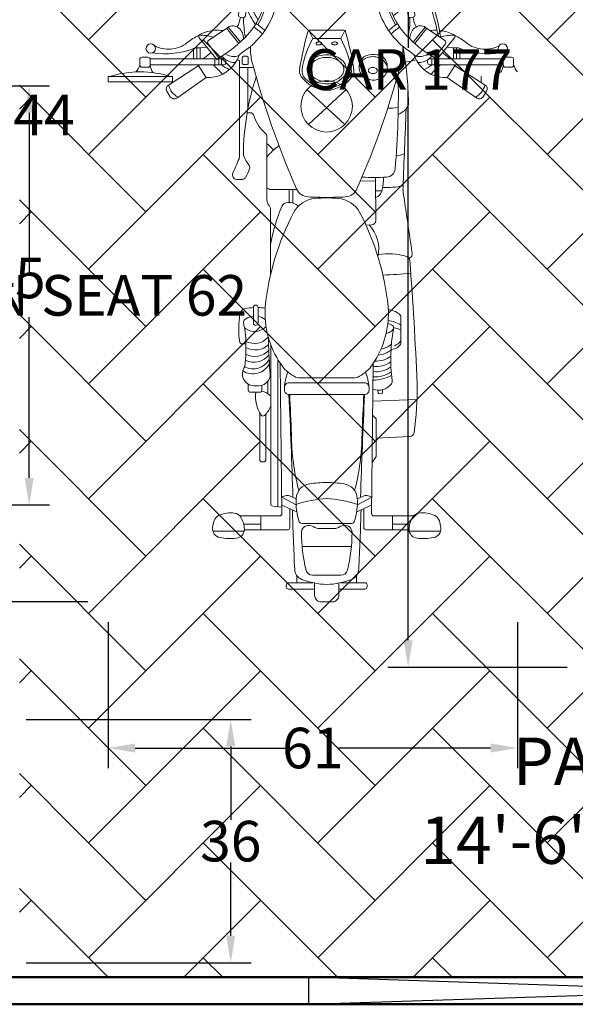
# Model space of a CAD drawing. Units: inches. Extents: x -466983 to 1020, y 324 to 318697.
# Tile 23 of 97: x 814 to 896, y 365 to 511. Entities that reach past the tile are written whole.
import ezdxf

# ---------------------------------------------------------------- set-up
doc = ezdxf.new("R2010")
doc.units = ezdxf.units.IN
doc.header["$MEASUREMENT"] = 0
for name, color, linetype, lineweight in [('A-ANNO-DIMS', 2, 'Continuous', 18), ('A-AREA-IDEN', 7, 'Continuous', 25), ('A-DOOR', 3, 'Continuous', 25), ('A-EQPM-VEHC', 8, 'Continuous', 18), ('A-FLOR-PATT', 252, 'Continuous', 13), ('A-WALL', 7, 'Continuous', 50)]:
    doc.layers.add(name, color=color, linetype=linetype, lineweight=lineweight)
doc.styles.get("Standard").update_dxf_attribs({"font": 'arial.ttf'})
doc.dimstyles.get("Standard").update_dxf_attribs({"dimtxt": 6, "dimasz": 4, "dimexe": 3, "dimexo": 3, "dimgap": 0.09, "dimtad": 0, "dimtih": 1, "dimtoh": 1, "dimdec": 1, "dimzin": 0, "dimdsep": 46, "dimlunit": 3, "dimtxsty": 'Standard', "dimcen": 0.09, "dimadec": 0, "dimazin": 0, "dimtfac": 1, "dimtdec": 1, "dimtofl": 0, "dimtmove": 0, "dimatfit": 3, "dimfxl": 1, "dimtolj": 1, "dimtzin": 0, "dimarcsym": 0})

# ---------------------------------------------------------------- blocks, each defined once
blk = doc.blocks.new('Bike')
for p, q in [((3716.6, 1477), (3739.4, 1477)), ((3715, 1462.6), (3739.4, 1462.6)), ((3715.3, 1469.7), (3739.4, 1469.7)), ((3725.9, 1437.8), (3739.4, 1455.6)), ((3476.2, 1372.3), (3476.2, 1447.6)), ((3479.4, 1371.4), (3479.4, 1449.1)), ((4796.8, 1363.8), (4796.8, 1434.1)), ((3739.4, 1429.3), (3753.1, 1429.3)), ((3739.4, 1420.3), (3753.1, 1420.3)), ((3739.4, 1414.7), (3753.1, 1414.7)), ((3511.5, 1359.9), (3511.5, 1390.3)), ((3668.6, 1399.5), (3702.1, 1372.5)), ((3671.4, 1403.4), (3705.4, 1376.1)), ((3478.1, 1297.1), (3478.1, 1372)), ((3491.8, 1338.1), (3491.8, 1373.1)), ((4502.2, 1381), (4505.8, 1282.1)), ((3511.5, 1346.8), (3511.5, 1327.3)), ((4781.5, 1364.7), (4781.5, 1326.4)), ((3478.1, 1338.1), (3495.7, 1338.1)), ((3505.6, 1338.1), (3511.5, 1338.1)), ((4762.6, 1326.4), (4793.8, 1326.4)), ((4035.1, 1288.5), (4035.1, 1302.5)), ((3491.8, 1289.6), (3530.3, 1289.6)), ((4012.9, 1254.3), (4013.4, 1288.4)), ((4721.1, 1279.7), (4737.7, 1247.6)), ((4738.5, 1279.5), (4753.4, 1246.1)), ((3106.7, 1249.4), (3106.7, 1240.7)), ((3129.5, 1249.4), (3129.5, 1240.7)), ((3460.4, 1251.7), (3510.3, 1251.7)), ((3517.1, 1251.6), (3529.2, 1251.6)), ((3542.4, 1251.6), (3546.2, 1251.6)), ((4896.6, 1245.7), (4912.2, 1245.7)), ((3808.6, 1222.8), (3886.6, 1138)), ((3808.6, 1134.7), (3886.6, 1219.4)), ((3489.4, 1202.6), (3538.3, 1202.6)), ((3489.4, 1155.3), (3538.3, 1155.3)), ((3676.5, 1138.6), (3694.4, 1147.6)), ((3106.7, 1108.5), (3106.7, 1117.1)), ((3129.5, 1108.5), (3129.5, 1117.1)), ((3460.4, 1106.2), (3510.3, 1106.2)), ((3517.1, 1106.2), (3529.2, 1106.2)), ((3542.4, 1106.2), (3546.2, 1106.2)), ((4032.4, 1103.3), (4062.6, 1103.3)), ((4721.1, 1078.2), (4737.7, 1110.3)), ((4738.5, 1078.4), (4753.4, 1111.8)), ((4896.6, 1112.2), (4912.2, 1112.2)), ((4032.4, 1094.9), (4061.1, 1094.9)), ((3478.1, 1060.8), (3478.1, 985.9)), ((3491.8, 1068.2), (3530.3, 1068.2)), ((4412.5, 1069.2), (4742.2, 1069.2)), ((4461.5, 1046.8), (4489.1, 1046.8)), ((3478.1, 1019.8), (3500.2, 1019.8)), ((3491.8, 1019.8), (3491.8, 984.8)), ((3500.1, 1019.8), (3511.5, 1019.8)), ((3511.5, 996.5), (3511.5, 1030.6)), ((3758.9, 1015.1), (3758.9, 983.2)), ((4762.6, 1031.4), (4793.8, 1031.4)), ((4781.5, 993.1), (4781.5, 1031.4)), ((3511.5, 998), (3511.5, 967.6)), ((3758.9, 1002.4), (3851.5, 1002.4)), ((4796.8, 994.1), (4796.8, 923.8)), ((3476.2, 985.5), (3476.2, 910.3)), ((3479.4, 986.4), (3479.4, 908.8)), ((3668.6, 958.4), (3702.1, 985.4)), ((3671.4, 954.4), (3705.4, 981.8)), ((3739.4, 943.1), (3753.1, 943.1)), ((3739.4, 937.5), (3753.1, 937.5)), ((3739.4, 928.6), (3753.1, 928.6)), ((3725.9, 920.1), (3739.4, 902.3)), ((3755, 891.8), (3781.3, 909.1)), ((3715, 895.3), (3739.4, 895.3)), ((3715.3, 888.2), (3739.4, 888.2)), ((3716.6, 880.8), (3739.4, 880.8))]:
    blk.add_line(p, q)
for points in [[(3736.2, 1579.4), (3736.2, 1592.7, -0.414214), (3741.2, 1597.7), (3753.5, 1597.7, -0.414214), (3758.5, 1592.7), (3758.5, 1579.4, -0.414214), (3753.5, 1574.4), (3741.2, 1574.4, -0.414214)], [(3506.4, 1438.1, 0.044309), (3491.8, 1448.2, 0.12965), (3486.9, 1449.5), (3482.3, 1449.5, 0.116215), (3477.8, 1448.5, 0.026021), (3471.7, 1445, 0.256394), (3464.8, 1432.4), (3464.8, 1387.3, 0.252462), (3471.5, 1374.8, 0.012105), (3473, 1373.9, 0.288965), (3494.3, 1374.5, 0.06955), (3510.2, 1388.8, 0.177075), (3517.3, 1408.1), (3517.3, 1415, 0.223082)], [(4811.1, 1418.6, 0.390363), (4789.3, 1434.7, 0.055736), (4773.5, 1431.2, 0.196303), (4762.1, 1421.2, 0.154867), (4756.5, 1385.4, 0.215074), (4765.4, 1371.6, 0.140504), (4792.5, 1363.4, 0.387027), (4812.7, 1381.2, 0.07489)], [(3764.2, 1314.8, 0.116891), (3754.2, 1313.4, 0.104306), (3744.8, 1307.4, 0.090357), (3738.3, 1297.9, 0.08248), (3735, 1285.8, 0.08248), (3735.8, 1273.2, 0.090357), (3740.4, 1262.7, 0.104306), (3748.4, 1254.9, 0.116891), (3757.9, 1251.6, 0.116891), (3767.8, 1252.9, 0.104306), (3777.2, 1259, 0.090357), (3783.8, 1268.4, 0.08248), (3787.1, 1280.6, 0.08248), (3786.2, 1293.1, 0.090357), (3781.7, 1303.7, 0.104306), (3773.6, 1311.5, 0.116891)], [(4294.6, 1316.7, 0.093727), (4084.2, 1253.4, 0.26048), (4052.1, 1204.4, 0.011277), (4050.8, 1178.9, 0.011277), (4052.1, 1153.4, 0.26048), (4084.2, 1104.5, 0.093727), (4294.6, 1041.2, 0.168473), (4422.7, 1075.8, 0.123184), (4450.3, 1105.7, 0.12588), (4454, 1120.1), (4454, 1178.9), (4454, 1237.8, 0.12588), (4450.3, 1252.2, 0.123184), (4422.7, 1282.1, 0.168473)], [(3564.6, 1285.6, 0.137096), (3561.5, 1285.3, 0.107007), (3558.1, 1283.1, 0.081077), (3555.6, 1279.7, 0.06906), (3554.1, 1275, 0.06906), (3553.9, 1270, 0.081077), (3554.9, 1265.9, 0.107007), (3557.3, 1262.7, 0.137096), (3560.1, 1261.3, 0.137096), (3563.3, 1261.6, 0.107007), (3566.7, 1263.8, 0.081077), (3569.1, 1267.2, 0.06906), (3570.7, 1271.9, 0.06906), (3570.9, 1276.8, 0.081077), (3569.8, 1280.9, 0.107007), (3567.5, 1284.2, 0.137096)], [(3766.3, 1292.1, 0.136763), (3763.8, 1291.6, 0.10699), (3761.3, 1289.5, 0.081228), (3759.7, 1286.4, 0.069255), (3758.9, 1282.5, 0.069255), (3759.2, 1278.5, 0.081228), (3760.5, 1275.3, 0.10699), (3762.8, 1272.9, 0.136763), (3765.2, 1272.1, 0.136763), (3767.7, 1272.7, 0.10699), (3770.2, 1274.8, 0.081228), (3771.8, 1277.8, 0.069255), (3772.6, 1281.8, 0.069255), (3772.3, 1285.8, 0.081228), (3771, 1288.9, 0.10699), (3768.7, 1291.3, 0.136763)], [(3409.7, 1259.3, 0.088306), (3400.8, 1259.5, 0.265111), (3393, 1253.4, 0.077673), (3375.4, 1178.9, 0.077673), (3393, 1104.4, 0.265111), (3400.8, 1098.3, 0.088306), (3409.7, 1098.6, 0.355135), (3417.6, 1108.4), (3417.6, 1178.9), (3417.6, 1249.5, 0.355135)], [(3556.1, 1227.7), (3556.1, 1236.5, -0.414214), (3561.1, 1241.5), (3613.3, 1241.5, -0.414214), (3618.3, 1236.5), (3618.3, 1227.7, -0.414214), (3613.3, 1222.7), (3561.1, 1222.7, -0.414214)], [(3779.6, 1236, 0.198787), (3764.7, 1239.7, 0.033352), (3679.3, 1221.3, 0.334742), (3675.6, 1216.5), (3675.6, 1178.9), (3675.6, 1141.3, 0.334742), (3679.3, 1136.5, 0.033352), (3764.7, 1118.1, 0.198787), (3779.6, 1121.9, 0.220896), (3810.5, 1178.9, 0.220896)], [(4687.9, 1178.9, 0.027846), (4690.9, 1140.7, 0.357798), (4723.4, 1110.4, 0.096715), (4776.1, 1117.3, 0.32255), (4779.5, 1122.1), (4779.5, 1178.9), (4779.5, 1235.8, 0.32255), (4776.1, 1240.6, 0.096715), (4723.4, 1247.4, 0.357798), (4690.9, 1217.2, 0.027846)], [(4790.8, 1178.9), (4790.8, 1160.8, -0.145244), (4788.4, 1152.6, 0.168226), (4784.2, 1135.8, 0.389485), (4799.2, 1122.2, 0.058321), (4883.9, 1132.5, 0.346221), (4895.4, 1147.1), (4895.4, 1178.9), (4895.4, 1210.8, 0.346221), (4883.9, 1225.4, 0.058321), (4799.2, 1235.7, 0.389485), (4784.2, 1222, 0.168226), (4788.4, 1205.3, -0.145244), (4790.8, 1197.1)], [(3730.6, 1178.9, 0.074545), (3733.2, 1161.5, 0.085152), (3740.2, 1147.8, 0.106245), (3751.3, 1138, 0.128192), (3763.2, 1134.9, 0.128192), (3775.2, 1138, 0.106245), (3786.3, 1147.8, 0.085152), (3793.3, 1161.5, 0.074545), (3795.9, 1178.9, 0.074545), (3793.3, 1196.3, 0.085152), (3786.3, 1210.1, 0.106245), (3775.2, 1219.9, 0.128192), (3763.2, 1223, 0.128192), (3751.3, 1219.9, 0.106245), (3740.2, 1210.1, 0.085152), (3733.2, 1196.3, 0.074545)], [(3736.5, 1178.9, 0.070978), (3738.7, 1163.7, 0.082547), (3744.4, 1151.7, 0.106804), (3753.7, 1143.1, 0.13387), (3763.6, 1140.5, 0.13387), (3773.4, 1143.1, 0.106804), (3782.7, 1151.7, 0.082547), (3788.4, 1163.7, 0.070978), (3790.6, 1178.9, 0.070978), (3788.4, 1194.2, 0.082547), (3782.7, 1206.1, 0.106804), (3773.4, 1214.7, 0.13387), (3763.6, 1217.4, 0.13387), (3753.7, 1214.7, 0.106804), (3744.4, 1206.1, 0.082547), (3738.7, 1194.2, 0.070978)], [(3705.3, 1202.8, 0.162281), (3704.1, 1202.4, 0.10607), (3702.8, 1200.9, 0.070038), (3702.1, 1199, 0.056281), (3701.8, 1196.5, 0.056281), (3702.1, 1194, 0.070038), (3702.8, 1192.1, 0.10607), (3704.1, 1190.7, 0.162281), (3705.3, 1190.3, 0.162281), (3706.5, 1190.7, 0.10607), (3707.7, 1192.1, 0.070038), (3708.4, 1194, 0.056281), (3708.7, 1196.5, 0.056281), (3708.4, 1199, 0.070038), (3707.7, 1200.9, 0.10607), (3706.5, 1202.4, 0.162281)], [(3705.3, 1155.1, 0.162281), (3706.5, 1155.5, 0.10607), (3707.7, 1156.9, 0.070038), (3708.4, 1158.8, 0.056281), (3708.7, 1161.4, 0.056281), (3708.4, 1163.9, 0.070038), (3707.7, 1165.8, 0.10607), (3706.5, 1167.2, 0.162281), (3705.3, 1167.6, 0.162281), (3704.1, 1167.2, 0.10607), (3702.8, 1165.8, 0.070038), (3702.1, 1163.9, 0.056281), (3701.8, 1161.4, 0.056281), (3702.1, 1158.8, 0.070038), (3702.8, 1156.9, 0.10607), (3704.1, 1155.5, 0.162281)], [(3556.1, 1130.2), (3556.1, 1121.4, 0.414214), (3561.1, 1116.4), (3613.3, 1116.4, 0.414214), (3618.3, 1121.4), (3618.3, 1130.2, 0.414214), (3613.3, 1135.2), (3561.1, 1135.2, 0.414214)], [(3564.6, 1072.3, 0.137096), (3567.5, 1073.7, 0.107007), (3569.8, 1077, 0.081077), (3570.9, 1081, 0.06906), (3570.7, 1086, 0.06906), (3569.1, 1090.7, 0.081077), (3566.7, 1094.1, 0.107007), (3563.3, 1096.3, 0.137096), (3560.1, 1096.6, 0.137096), (3557.3, 1095.2, 0.107007), (3554.9, 1091.9, 0.081077), (3553.9, 1087.9, 0.06906), (3554.1, 1082.9, 0.06906), (3555.6, 1078.2, 0.081077), (3558.1, 1074.8, 0.107007), (3561.5, 1072.6, 0.137096)], [(4291, 1019.6), (4291, 1020, -0.414214), (4296, 1025), (4331.3, 1025, -0.414214), (4336.3, 1020), (4336.3, 1019.6, -0.414214), (4331.3, 1014.6), (4296, 1014.6, -0.414214)], [(3734.1, 992.8), (3734.1, 999.9, -0.414214), (3737.1, 1002.9), (3749.4, 1002.9, -0.414214), (3752.4, 999.9), (3752.4, 992.8, -0.414214), (3749.4, 989.8), (3737.1, 989.8, -0.414214)], [(4812.7, 976.7, 0.387027), (4792.5, 994.5, 0.140504), (4765.4, 986.3, 0.215074), (4756.5, 972.5, 0.154867), (4762.1, 936.7, 0.196303), (4773.5, 926.7, 0.055736), (4789.3, 923.2, 0.390363), (4811.1, 939.2, 0.07489)], [(3517.3, 942.8), (3517.3, 949.8, 0.177075), (3510.2, 969.1, 0.06955), (3494.3, 983.4, 0.288965), (3473, 984, 0.012105), (3471.5, 983.1, 0.252462), (3464.8, 970.6), (3464.8, 925.5, 0.256394), (3471.7, 912.9, 0.026021), (3477.8, 909.4, 0.116215), (3482.3, 908.4), (3486.9, 908.4, 0.12965), (3491.8, 909.7, 0.044309), (3506.4, 919.8, 0.223082)], [(3780.1, 689), (3790, 689, 0.414214), (3791, 690), (3791, 832.2, 0.414214), (3790, 833.2), (3780.1, 833.2, 0.414214), (3779.1, 832.2), (3779.1, 690, 0.414214)], [(3736.2, 778.4), (3736.2, 765.2, 0.414214), (3741.2, 760.2), (3753.5, 760.2, 0.414214), (3758.5, 765.2), (3758.5, 778.4, 0.414214), (3753.5, 783.4), (3741.2, 783.4, 0.414214)]]:
    blk.add_lwpolyline(points, format="xyb", close=True)
for points in [[(3713.9, 1447.6, 0.022793), (3715.3, 1473.8, 0.136), (3726.4, 1569.3)], [(3739.4, 1574.8), (3739.4, 1409.9, 0.414214), (3744.4, 1404.9), (3748.1, 1404.9, 0.414214), (3753.1, 1409.9), (3753.1, 1574.4)], [(3691, 1434, -0.079005), (3686.9, 1465, -0.05973), (3703.5, 1491.3, 0.159047), (3718.1, 1528.9, 0.126021), (3710.9, 1564.4)], [(3753.1, 1463), (3798.3, 1533.8, -0.40834), (3811.9, 1536.9), (3824.4, 1529.3, -0.431541), (3827.4, 1515.1), (3781.3, 1448.7), (3755, 1466.1)], [(3779.1, 1525.7, 0.414214), (3780.1, 1524.7), (3790, 1524.7, 0.414214), (3791, 1525.7)], [(3742, 1424.6), (3692.9, 1464.8, 0.483058), (3685.2, 1463.1, 0.088789), (3676.2, 1431.5)], [(3692.5, 1434.2, 0.096183), (3535.6, 1379.4, 0.22037), (3483.3, 1302.5)], [(3579.8, 1394.4), (3579.8, 1391.2, 0.349421), (3583.7, 1386.3, 0.057073), (3613.1, 1383, 0.413662), (3618.1, 1388), (3618.1, 1433.9, 0.414214), (3613.1, 1438.9), (3594.8, 1438.9, 0.414214), (3579.8, 1423.9), (3579.8, 1401.9)], [(3737.5, 1420.6), (3706.2, 1444.8, 0.431039), (3699, 1443.7), (3669.3, 1400.5, 0.337774), (3670.5, 1376.2, 0.230362), (3695.1, 1365.4)], [(3741.3, 1406, -0.159938), (3748.2, 1383.3, 0.280919), (3781.3, 1448.7)], [(3688.4, 1428.2, 0.089404), (3543.1, 1375.3, 0.184983), (3494.2, 1313)], [(3537.7, 1208.8, -0.564837), (3504.3, 1226.3, -0.102735), (3505.1, 1243.5, -0.140154), (3509.2, 1250.6, -0.082892), (3602.5, 1314.4, -0.053437), (3615.6, 1318.8, 0.151196), (3693.3, 1363.4, 0.070423), (3739.4, 1423.8)], [(3603.7, 1241.5), (3603.7, 1249.5, -0.101252), (3612.6, 1280.5, -0.13244), (3623.3, 1292, -0.090169), (3638.2, 1297.9, 0.164837), (3725.3, 1368), (3729.9, 1373.3, 0.174158), (3734.8, 1386, 0.159727), (3728.6, 1406.2)], [(3454.1, 1241.7, -0.235435), (3643.3, 1361.2, 0.410863), (3647.8, 1366.7, 0.044254), (3646.7, 1372.8, 0.360214), (3641.5, 1376.5, 0.253572), (3442.6, 1247.5)], [(3851.8, 1356.9, 0.001252), (4028.5, 1349.8, 0.046276), (4039.5, 1350.4, 0.000101), (4174.5, 1370.4, -0.314799), (4184.8, 1365.3), (4186, 1363.2)], [(4589, 1290), (4585.2, 1365.1, 0.35984), (4576.7, 1374.5, 0.038725), (4466.4, 1381.4, 0.009033), (4191, 1365, 0.303597), (4182.3, 1358.1, 0.12706), (4178.4, 1294.5)], [(4421.3, 1283), (4757.5, 1279.3, 0.417467), (4762.6, 1284.3), (4762.6, 1373.6)], [(3711.6, 1008.5, 0.070303), (3742.4, 1010.7, 0.039628), (4030.9, 1111.4, 0.282444), (4048.7, 1137.2, 0.015247), (4049.8, 1178.9, 0.015247), (4048.7, 1220.7, 0.282444), (4030.9, 1246.5, 0.039628), (3742.4, 1347.2, 0.070303), (3711.6, 1349.4)], [(3864.3, 1338.9, 0.080734), (3852.8, 1356, 0.212509), (3837.8, 1362.2, 0.038096), (3711.9, 1349.7)], [(4301, 1317, -0.138428), (4310.6, 1341, -0.233155), (4318.5, 1344.9), (4374.8, 1344.9, -0.216687), (4382.4, 1341.5, -0.156826), (4390.4, 1322.8)], [(4746.4, 1261.7), (4788.8, 1261.7, 0.414214), (4793.8, 1266.7), (4793.8, 1363.4)], [(4004.7, 1257.8, 0.018709), (4004.5, 1312.9, 0.375923), (3986.3, 1332, 0.029426), (3773.7, 1338.7)], [(4354.1, 1312.1, 0.056144), (4350.9, 1321, 0.085082), (4347.3, 1326.2, 0.153535), (4342.4, 1328.6, 0.197677), (4338.3, 1327.7, 0.1268), (4335.1, 1324, 0.072333), (4332.4, 1315.8, 0.051836)], [(4479.1, 1282.4, 0.326046), (4467.3, 1323.7, 0.2025), (4459.8, 1325.7, -0.079204), (4344.5, 1328.2)], [(3611.5, 1313.2, 0.084453), (3515.3, 1250, 0.185223), (3510.6, 1240.3, 0.080228), (3511.8, 1223.9, 0.449113), (3537, 1214.3)], [(3627.1, 1321.9, 0.043315), (3622.3, 1319.9, 0.279952), (3580.6, 1252.4), (3580.6, 1241.5)], [(3757.9, 1314.5, 0.058653), (3749, 1313.6, 0.314496), (3730.4, 1291.7, 0.11242), (3732.3, 1267.9, 0.161441), (3739.7, 1257.7, 0.088312), (3749.1, 1253.2, 0.094137), (3758.6, 1251.5)], [(4050.2, 1288.6, 0.000873), (4050.2, 1288.7, 0.265813), (4035.8, 1302.3, 0.056152), (4004.7, 1306.3)], [(4481.3, 1293.5), (4486.7, 1293.8, 0.420229), (4488.6, 1296), (4488.1, 1302.3, 0.415516), (4485.9, 1304.1), (4480.3, 1303.7)], [(3284.5, 1297.1), (3100.9, 1297.1, 0.226605), (3093.1, 1293.4, 0.400758), (3096.5, 1251.9, 0.183413), (3103.2, 1249.4), (3281.2, 1249.4)], [(3324.7, 1299.2, 0.006041), (3316.2, 1299.3), (3290.7, 1299.3, 0.172401), (3284.4, 1297, 0.450807), (3282.4, 1248.2, 0.193514), (3289.3, 1245.4), (3311, 1245.4, 0.017498), (3327.2, 1245.7)], [(3334.2, 1289.8, 0.161741), (3331.4, 1296.9, 0.157572), (3325.7, 1299, 0.171418), (3320.4, 1297.4, 0.113331), (3316.3, 1292.6, 0.072079), (3313, 1283.4, 0.055689), (3312.2, 1273.3, 0.053775), (3313.6, 1263, 0.064911), (3317.3, 1253.4, 0.09694), (3321.7, 1248.1, 0.155824), (3327.4, 1245.9, 0.172526), (3332.7, 1247.4, 0.151352), (3336.2, 1251.6)], [(3392.3, 1251.6), (3324.6, 1251.6, -0.26356), (3320.3, 1254, -0.214715), (3316.5, 1286.3, -0.327171), (3321.3, 1289.8), (3471.6, 1289.8)], [(3570.1, 1297.2, 0.144644), (3549.1, 1299.6, 0.369621), (3527.5, 1282.5, 0.036315), (3527.3, 1266.8)], [(3555, 1300.1, 0.253732), (3540.7, 1282.5, 0.012512), (3540.3, 1277.1)], [(3541.9, 1253.9, 0.31484), (3574.9, 1255.4, 0.193965), (3580.6, 1265, 0.061634), (3581.2, 1286.2, 0.219833), (3576.9, 1293.4, 0.014528), (3575.1, 1294.6)], [(4005.1, 1288.4), (4101.4, 1288.7, -0.407202), (4111.4, 1279), (4111.7, 1266.7)], [(4720.8, 1279.7, 0.108929), (4717, 1269, 0.145286), (4718.3, 1260.6), (4724.6, 1247.5)], [(3527.8, 1096.9, -0.055925), (3533.1, 1120.5, 0.050281), (3539.5, 1178.9, 0.050281), (3533.1, 1237.4, -0.055925), (3527.8, 1261)], [(3540.3, 1086.8, -0.079272), (3546.2, 1120.5, 0.050281), (3552.6, 1178.9, 0.050281), (3546.2, 1237.4, -0.079272), (3540.3, 1271.1)], [(4721.2, 1103.2, 0.004418), (4491.2, 1094.2, -0.414214), (4481.2, 1084.2), (4474.7, 1084.2, -0.414214), (4464.7, 1094.2), (4464.7, 1178.9), (4464.7, 1263.7, -0.414214), (4474.7, 1273.7), (4481.2, 1273.7, -0.414214), (4491.2, 1263.7)], [(4491.2, 1094.2), (4491.2, 1178.9), (4491.2, 1263.7, 0.004418), (4721.2, 1254.7)], [(4705.9, 1241.5, 0.063368), (4580, 1258, -0.001705), (4491.2, 1262)], [(4926.4, 1206.2), (4926.4, 1264.5, 0.414214), (4921.4, 1269.5), (4917.2, 1269.5, 0.414214), (4912.2, 1264.5), (4912.2, 1210.4)], [(3388.2, 1117.1), (3071.5, 1117.1, -0.369002), (3046.8, 1138.2, -0.033307), (3043.1, 1178.9, -0.033307), (3046.8, 1219.6, -0.369002), (3071.5, 1240.7), (3388.2, 1240.7)], [(3392.7, 1239.9, 0.062968), (3380.1, 1178.9, 0.062968), (3392.7, 1118)], [(3416.3, 1103.3, 0.231711), (3486.9, 1148.9, 0.086055), (3494.3, 1178.9, 0.086055), (3486.9, 1209, 0.231711), (3416.3, 1254.6)], [(3694.4, 1210.2), (3694.4, 1178.9), (3694.4, 1147.6, 0.084607), (3762, 1124, 0.24184), (3783.8, 1130.9, 0.177565), (3806.3, 1178.9, 0.177565), (3783.8, 1227, 0.24184), (3762, 1233.9, 0.084607), (3694.4, 1210.2), (3676.5, 1219.3)], [(4736.9, 1247.6, 0.067766), (4724, 1178.9, 0.067766), (4736.9, 1110.2)], [(4748.9, 1102, 0.004183), (4881.9, 1107.1, 0.304225), (4904.8, 1123, 0.085326), (4916.2, 1178.9, 0.085326), (4904.8, 1234.8, 0.304225), (4881.9, 1250.8, 0.004183), (4748.9, 1255.9)], [(3551.4, 1136.8, 0.036141), (3554.8, 1178.9, 0.036141), (3551.4, 1221.1)], [(3608.7, 1135.2, -0.133909), (3615.9, 1165.1, 0.12166), (3620.2, 1178.9, 0.12166), (3615.9, 1192.7, -0.133909), (3608.7, 1222.7)], [(4913.1, 1206.2), (4940.3, 1206.2, -0.414214), (4955.3, 1191.2), (4955.3, 1178.9), (4955.3, 1166.7, -0.414214), (4940.3, 1151.7), (4913.1, 1151.7)], [(3537.7, 1149.1, 0.564837), (3504.3, 1131.6, 0.102735), (3505.1, 1114.4, 0.140154), (3509.2, 1107.3, 0.082892), (3602.5, 1043.5, 0.053437), (3615.6, 1039, -0.151196), (3693.3, 994.4, -0.070423), (3739.4, 934)], [(4912.2, 1147.5), (4912.2, 1093.4, 0.414214), (4917.2, 1088.4), (4921.4, 1088.4, 0.414214), (4926.4, 1093.4), (4926.4, 1151.7)], [(3537, 1143.6, 0.449113), (3511.8, 1134, 0.080228), (3510.6, 1117.6, 0.185223), (3515.3, 1107.9, 0.084453), (3611.5, 1044.6)], [(3281.2, 1108.5), (3103.2, 1108.5, 0.183413), (3096.5, 1106, 0.400758), (3093.1, 1064.5, 0.226605), (3100.9, 1060.7), (3284.5, 1060.7)], [(3327.2, 1112.1, 0.017498), (3311, 1112.5), (3289.3, 1112.5, 0.193514), (3282.4, 1109.7, 0.450807), (3284.4, 1060.8, 0.172401), (3290.7, 1058.6), (3316.2, 1058.6, 0.006041), (3324.7, 1058.7)], [(3336.2, 1106.3, 0.151352), (3332.7, 1110.5, 0.172526), (3327.4, 1112, 0.155824), (3321.7, 1109.8, 0.09694), (3317.3, 1104.4, 0.064911), (3313.6, 1094.9, 0.053775), (3312.2, 1084.5, 0.055689), (3313, 1074.5, 0.072079), (3316.3, 1065.2, 0.113331), (3320.4, 1060.5, 0.171418), (3325.7, 1058.8, 0.157572), (3331.4, 1060.9, 0.161741), (3334.2, 1068.1)], [(3392.3, 1106.3), (3324.6, 1106.3, 0.26356), (3320.3, 1103.8, 0.214715), (3316.5, 1071.6, 0.327171), (3321.3, 1068.1), (3471.6, 1068.1)], [(3442.6, 1110.3, 0.253572), (3641.5, 981.4, 0.360214), (3646.7, 985.1, 0.044254), (3647.8, 991.2, 0.410863), (3643.3, 996.6, -0.235435), (3454.1, 1116.2)], [(3575.1, 1063.2, 0.014528), (3576.9, 1064.4, 0.219833), (3581.2, 1071.7, 0.061634), (3580.6, 1092.8, 0.193965), (3574.9, 1102.5, 0.31484), (3541.9, 1104)], [(3580.6, 1116.4), (3580.6, 1105.5, 0.279952), (3622.3, 1037.9, 0.043315), (3627.1, 1036)], [(3728.6, 951.6, 0.159727), (3734.8, 971.9, 0.174158), (3729.9, 984.5), (3725.3, 989.8, 0.164837), (3638.2, 1059.9, -0.090169), (3623.3, 1065.9, -0.13244), (3612.6, 1077.3, -0.101252), (3603.7, 1108.3), (3603.7, 1116.4)], [(4032.4, 1112), (4032.4, 1054.3, -0.140419), (4030.9, 1049), (4028.4, 1045)], [(4069.3, 1115.5, 0.182977), (4061, 1091.7, 0.292151), (4070, 1078.3, 0.060635), (4155.6, 1053.1)], [(4491.2, 1095.9, -0.001705), (4580, 1099.9, 0.063368), (4705.9, 1116.4)], [(4724.6, 1110.4), (4718.3, 1097.3, 0.145286), (4717, 1088.8, 0.108929), (4720.8, 1078.2)], [(3527.3, 1091.1, 0.036315), (3527.5, 1075.3, 0.369621), (3549.1, 1058.3, 0.144644), (3570.1, 1060.7)], [(3540.3, 1080.8, 0.012512), (3540.7, 1075.3, 0.253732), (3555, 1057.8)], [(4793.8, 994.5), (4793.8, 1091.2, 0.414214), (4788.8, 1096.2), (4746.4, 1096.2)], [(4379.8, 1053.5), (4735.9, 1053.5, 0.378085), (4740.8, 1057.9), (4743.4, 1078.4)], [(4762.6, 984.3), (4762.6, 1073.6, 0.417467), (4757.5, 1078.6), (4421.3, 1074.8)], [(3860.2, 1000.8), (3860.2, 1006.9, -0.339938), (3867.7, 1016.5, 0.159134), (3905.8, 1041.3, -0.226589), (3913.5, 1045), (4055.5, 1045, 0.174252), (4068.2, 1049.6), (4069.7, 1050.8, -0.174252), (4076, 1053.1), (4223.9, 1053.1)], [(4316, 1014.6, 0.114491), (4321.5, 997.6, 0.239101), (4329.2, 992.8, 0.103983), (4339, 994, 0.167173), (4344.1, 997.9, 0.363558), (4338.9, 1042.9)], [(4338.2, 993.7, -0.040508), (4365, 997.7, -0.03842), (4428.6, 995.4, 0.607774), (4471.6, 1015.9), (4471.5, 1027, 0.485016), (4437.8, 1051.6, -0.00298), (4362, 1047.8)], [(4485.9, 1020.1, 0.170118), (4536.9, 1031.7, 0.477675), (4537.8, 1039.4, 0.09469), (4517.6, 1053.5)], [(4532, 1028.9), (4637, 1028.9, 0.414214), (4642, 1033.9), (4642, 1037.6, 0.414214), (4637, 1042.6), (4534.5, 1042.6)], [(3741.8, 978.4, 0.005304), (3743.1, 983.2), (3959.4, 983.2, -0.102096), (3963.4, 982.4, 0.00244), (3995.8, 968.6, 0.501027), (4009.6, 976.7, 0.054221), (4009.7, 990, 0.228934), (4005.1, 997.3, 0.079407), (3985, 1006, 0.239312), (3976.1, 1004, -0.075874), (3957.8, 993, -0.0999), (3953.9, 992.2, -0.077513), (3779.8, 1020.9)], [(4296.5, 1014.6, 0.031683), (4298.6, 996.5, 0.319342), (4310.9, 984.3, 0.078645), (4373.6, 984.1, 0.339222), (4377.8, 988.5, 0.096684), (4377, 998)], [(4470.4, 1033.9), (4480.9, 1033.9, -0.414214), (4485.9, 1028.9), (4485.9, 1008.2, -0.414214), (4480.9, 1003.2), (4467.9, 1003.2)], [(3695.1, 992.5, 0.230362), (3670.5, 981.6, 0.337774), (3669.3, 957.4), (3699, 914.2, 0.431039), (3706.2, 913.1), (3737.5, 937.3)], [(3593, 990.1, 0.064082), (3595.5, 956.1, 0.274699), (3598.9, 952.4, 0.213807), (3609.1, 953.6, 0.217468), (3611.4, 957.1, 0.038755), (3614, 985.1)], [(3753.1, 894.9), (3798.3, 824.1, 0.40834), (3811.9, 820.9), (3824.4, 828.5, 0.431541), (3827.4, 842.8), (3781.3, 909.1, 0.280919), (3748.2, 974.6, -0.159938), (3741.3, 951.9)], [(3753.1, 783.4), (3753.1, 948, 0.414214), (3748.1, 953), (3744.4, 953, 0.414214), (3739.4, 948), (3739.4, 783.1)], [(3676.4, 947.1, 0.047742), (3675.9, 929.4), (3675.9, 929.3, 0.096803), (3685.2, 894.8, 0.483058), (3692.9, 893.1), (3742, 933.3)], [(3691.4, 925.3, 0.082553), (3686.9, 892.9, 0.05973), (3703.5, 866.6, -0.159047), (3718.1, 829, -0.126021), (3710.9, 793.5)], [(3726.4, 788.6, 0.136), (3715.3, 884.1, 0.022793), (3713.9, 910.3)]]:
    blk.add_lwpolyline(points, format="xyb")
for points in [[(4537.3, 1281.8), (4545.1, 1290), (4630.1, 1290), (4643.2, 1280.6)], [(3392.7, 1105.3), (3392.7, 1178.9), (3392.7, 1252.6)], [(4831, 1234.2), (4831, 1178.9), (4831, 1123.7)], [(3050.6, 1229.4), (2939.7, 1229.4), (2802.2, 1229.4), (2775.9, 1217), (2775.9, 1164.4)], [(2776, 1217), (2957.8, 1217), (3046.4, 1217)], [(3580.6, 1222.7), (3580.6, 1178.9), (3580.6, 1135.2)], [(3603.7, 1222.7), (3603.7, 1178.9), (3603.7, 1135.2)], [(3050.6, 1128.5), (2939.7, 1128.5), (2802.2, 1128.5), (2775.9, 1140.9), (2775.9, 1193.5)], [(2776, 1140.9), (2957.8, 1140.9), (3046.4, 1140.9)]]:
    blk.add_lwpolyline(points)
for centre, radius in [((3716.6, 1573.3), 10.6), ((3845.9, 1178.7), 57.6), ((3716.6, 784.6), 10.6)]:
    blk.add_circle(centre, radius)
for centre, radius, start, end in [((3741.5, 1637.1), 41.2, 286.9888, 312.0372), ((3749, 1534.6), 40.1, 57.3492, 83.449), ((3788.9, 1493.4), 40.9, 27.2359, 77.1495), ((3908.5, 1569.9), 206.8, 221.2614, 229.5793), ((3769, 1422), 93.3, 177.6075, 186.9102), ((3710.3, 1384.2), 37.9, 39.0272, 51.9723), ((3680.5, 1359.4), 91.4, 24.0671, 37.4396), ((3939.5, 1465.4), 346.6, 193.685, 195.7923), ((3803.7, 1426.1), 199.4, 192.4698, 195.6556), ((3774.2, 1434.7), 169, 197.8118, 201.3124), ((3639.5, 1433), 61.1, 276.8609, 298.2339), ((3711.2, 1436.9), 65.1, 287.813, 304.5915), ((3515.3, 1317.4), 234.8, 9.2486, 15.3175), ((3597.6, 1291.6), 626.2, 1.209, 6.9337), ((3939.5, 1465.4), 346.6, 198.4449, 204.6334), ((3803.7, 1426.1), 199.4, 200.2574, 210.9013), ((3774.2, 1434.7), 169, 206.8349, 219.1999), ((3649, 1152.2), 213.1, 78.6059, 90.3415), ((3923.3, 1335), 33.4, 359.0902, 32.2964), ((3841.7, 1313.3), 185.9, 357.1486, 11.3635), ((4387.6, 1310.4), 62.2, 146.2979, 174.4306), ((4408.7, 1315.7), 68.7, 154.8594, 169.0097), ((4355, 1321.8), 28.2, 18.3548, 54.9232), ((3584.9, 1462.7), 151.5, 283.3715, 301.3249), ((3834.7, 1458.1), 211.7, 214.8443, 221.5826), ((3842.4, 1463.3), 211.7, 214.9067, 221.5218), ((3733.5, 1322.4), 116.7, 356.6367, 8.2567), ((4337, 1290.1), 53.6, 11.0089, 38.6482), ((4349.2, 1289.8), 53.6, 4.6068, 37.9011), ((4362.7, 1290.1), 53.6, 356.0108, 36.9065), ((4374.9, 1290.1), 53.6, 352.3592, 36.9849), ((4386.5, 1290.4), 53.6, 351.8913, 37.1496), ((4388.7, 1287), 62.9, 356.0657, 35.4453), ((4364.1, 1281), 94.8, 0.9619, 27.161), ((3664.1, 1323.1), 52.9, 190.2344, 217.1371), ((3671.6, 1327), 52.9, 189.3206, 216.9338), ((3343.1, 1272.2), 42, 139.9272, 219.6749), ((3435.7, 1263), 41.9, 140.3451, 189.8858), ((3483.9, 1259.5), 69.2, 154.0504, 182.4153), ((3479.7, 1264.6), 43.4, 144.5037, 201.1055), ((3538.9, 1269.4), 45, 153.363, 203.2549), ((3783.3, 1235.1), 174.2, 162.8434, 177.8981), ((4165.8, 1215.8), 79.7, 77.8259, 132.9545), ((4481.9, 1161.8), 112.1, 93.7127, 111.5258), ((3394.4, 1259.4), 95.6, 334.4456, 355.3484), ((3397.9, 1258.1), 95.6, 333.0513, 356.1505), ((3585.6, 1280.9), 68.9, 237.8956, 265.8204), ((3394.4, 1098.5), 95.6, 4.6516, 25.5544), ((3397.9, 1099.8), 95.6, 3.8495, 26.9487), ((3585.6, 1077), 68.9, 94.1796, 122.1044), ((3343.1, 1085.7), 42, 140.3251, 220.0728), ((3435.7, 1094.9), 41.9, 170.1142, 219.6549), ((3479.7, 1093.3), 43.4, 158.8945, 215.4963), ((3538.9, 1088.4), 45, 156.7451, 206.637), ((3783.3, 1122.7), 174.2, 182.1019, 197.1566), ((3483.9, 1098.4), 69.2, 177.5847, 205.9496), ((4481.9, 1196.1), 112.1, 248.4742, 266.2873), ((3664.1, 1034.8), 52.9, 142.8629, 169.7656), ((3671.6, 1030.9), 52.9, 143.0662, 170.6794), ((4082.7, 908.2), 205.4, 132.3055, 138.2462), ((4027.2, 1133.1), 111.1, 213.3859, 232.4739), ((3584.9, 895.2), 151.5, 58.6751, 76.6285), ((3834.7, 899.8), 211.7, 138.4174, 145.1557), ((4440.3, 1021.4), 143.9, 172.1779, 178.584), ((4355.4, 1018.1), 39.6, 144.2076, 169.9356), ((4336.5, 1017), 40.3, 331.7508, 49.9014), ((4349.2, 1019.2), 42.2, 329.8767, 44.2278), ((4363.9, 1017.8), 42.2, 331.3167, 48.0597), ((4376.7, 1015.8), 42.2, 333.1337, 53.4177), ((4391.4, 1013.8), 42.2, 333.4944, 59.7642), ((4402.5, 1013.1), 42.2, 327.9971, 63.0183), ((4528.9, 1021.1), 47.3, 136.8041, 165.0837), ((3586.6, 1121.8), 117.1, 275.9386, 304.5183), ((3566.8, 1150.4), 162.3, 291.2356, 306.3114), ((3842.4, 894.6), 211.7, 138.4782, 145.0933), ((3649, 1205.7), 213.1, 269.6585, 281.3941), ((3639.5, 924.8), 61.1, 61.7661, 83.1391), ((3711.2, 921), 65.1, 55.4085, 72.187), ((3710.3, 973.7), 37.9, 308.0277, 320.9728), ((3680.5, 998.5), 91.4, 322.5604, 335.9329), ((3908.5, 788), 206.8, 130.4207, 138.7386), ((3788.9, 864.5), 40.9, 282.8505, 332.7641), ((4007, 761.1), 238.1, 163.1793, 196.8207), ((3749, 823.3), 40.1, 276.551, 302.6508), ((3741.5, 720.8), 41.2, 47.9628, 73.0112)]:
    blk.add_arc(centre, radius, start, end)
blk = doc.blocks.new('*D93')
at = {"layer": 'A-ANNO-DIMS', "color": 0, "lineweight": -2, "transparency": 16777216}
for p, q in [((808.97, 500.78), (818.27, 500.78)), ((815.27, 496.78), (815.27, 472.97)), ((815.27, 442.78), (815.27, 466.58)), ((808.97, 438.78), (818.27, 438.78))]:
    blk.add_line(p, q, dxfattribs=at)
at = {"layer": 'A-ANNO-DIMS', "color": 0, "transparency": 16777216}
for points in [[(814.6, 496.78), (815.93, 496.78), (815.27, 500.78)], [(814.6, 442.78), (815.93, 442.78), (815.27, 438.78)]]:
    blk.add_solid(points, dxfattribs=at)
at = {"layer": 'Defpoints', "color": 0, "transparency": 16777216}
for p in [(805.97, 500.78), (815.27, 500.78), (805.97, 438.78)]:
    blk.add_point(p, dxfattribs=at)
at = {"layer": 'A-ANNO-DIMS', "color": 0, "transparency": 16777216, "insert": (815.27, 469.78), "char_height": 6, "attachment_point": 5}
blk.add_mtext('\\A1;GARDEN SEAT 62', dxfattribs=at)
blk = doc.blocks.new('*D95')
at = {"layer": 'A-ANNO-DIMS', "color": 0, "lineweight": -2, "transparency": 16777216}
for p, q in [((894.88, 591.6), (868.36, 591.6)), ((871.36, 587.6), (871.36, 506.38)), ((871.36, 418.77), (871.36, 499.99)), ((894.88, 414.77), (868.36, 414.77))]:
    blk.add_line(p, q, dxfattribs=at)
at = {"layer": 'A-ANNO-DIMS', "color": 0, "transparency": 16777216}
for points in [[(870.69, 587.6), (872.03, 587.6), (871.36, 591.6)], [(870.69, 418.77), (872.03, 418.77), (871.36, 414.77)]]:
    blk.add_solid(points, dxfattribs=at)
at = {"layer": 'Defpoints', "color": 0, "transparency": 16777216}
for p in [(897.88, 591.6), (871.36, 414.77), (897.88, 414.77)]:
    blk.add_point(p, dxfattribs=at)
at = {"layer": 'A-ANNO-DIMS', "color": 0, "transparency": 16777216, "insert": (871.36, 503.18), "char_height": 6, "attachment_point": 5}
blk.add_mtext('\\A1;CAR 177', dxfattribs=at)
blk = doc.blocks.new('*D97')
at = {"layer": 'A-ANNO-DIMS', "color": 0, "lineweight": -2, "transparency": 16777216}
for p, q in [((823.93, 568.44), (802.33, 568.44)), ((805.33, 564.44), (805.33, 499.55)), ((805.33, 428.44), (805.33, 493.34)), ((823.93, 424.44), (802.33, 424.44))]:
    blk.add_line(p, q, dxfattribs=at)
at = {"layer": 'A-ANNO-DIMS', "color": 0, "transparency": 16777216}
for points in [[(804.66, 564.44), (806, 564.44), (805.33, 568.44)], [(804.66, 428.44), (806, 428.44), (805.33, 424.44)]]:
    blk.add_solid(points, dxfattribs=at)
at = {"layer": 'Defpoints', "color": 0, "transparency": 16777216}
for p in [(826.93, 568.44), (805.33, 424.44), (826.93, 424.44)]:
    blk.add_point(p, dxfattribs=at)
at = {"layer": 'A-ANNO-DIMS', "color": 0, "transparency": 16777216, "insert": (805.33, 496.44), "char_height": 6, "attachment_point": 5}
blk.add_mtext('\\A1;BIKE 144', dxfattribs=at)
blk = doc.blocks.new('*D98')
at = {"layer": 'A-ANNO-DIMS', "color": 0, "lineweight": -2, "transparency": 16777216}
for p, q in [((826.93, 421.44), (826.93, 399.84)), ((887.55, 421.44), (887.55, 399.84)), ((830.93, 402.84), (853.42, 402.84)), ((883.55, 402.84), (861.07, 402.84))]:
    blk.add_line(p, q, dxfattribs=at)
at = {"layer": 'A-ANNO-DIMS', "color": 0, "transparency": 16777216}
for points in [[(830.93, 403.51), (830.93, 402.17), (826.93, 402.84)], [(883.55, 403.51), (883.55, 402.17), (887.55, 402.84)]]:
    blk.add_solid(points, dxfattribs=at)
at = {"layer": 'Defpoints', "color": 0, "transparency": 16777216}
for p in [(826.93, 424.44), (887.55, 424.44), (887.55, 402.84)]:
    blk.add_point(p, dxfattribs=at)
at = {"layer": 'A-ANNO-DIMS', "color": 0, "transparency": 16777216, "insert": (857.24, 402.84), "char_height": 6, "attachment_point": 5}
blk.add_mtext('\\A1;61', dxfattribs=at)
blk = doc.blocks.new('*D113')
at = {"layer": 'A-ANNO-DIMS', "color": 0, "lineweight": -2, "transparency": 16777216}
for p, q in [((704.71, 504.65), (709.52, 509.41)), ((710.2, 504.46), (736.32, 478.05)), ((736.45, 472.55), (741.27, 477.31)), ((739.13, 475.2), (741.94, 472.36)), ((741.94, 472.36), (745.94, 472.36))]:
    blk.add_line(p, q, dxfattribs=at)
at = {"layer": 'A-ANNO-DIMS', "color": 0, "transparency": 16777216}
for points in [[(710.68, 504.93), (709.73, 503.99), (707.39, 507.3)], [(736.79, 478.52), (735.85, 477.58), (739.13, 475.2)]]:
    blk.add_solid(points, dxfattribs=at)
at = {"layer": 'Defpoints', "color": 0, "transparency": 16777216}
for p in [(702.58, 502.54), (739.13, 475.2), (734.32, 470.44)]:
    blk.add_point(p, dxfattribs=at)
at = {"layer": 'A-ANNO-DIMS', "color": 0, "transparency": 16777216, "insert": (783.5, 472.36), "char_height": 6, "attachment_point": 5}
blk.add_mtext('\\A1;TEA TABLE SET 45', dxfattribs=at)
blk = doc.blocks.new('*D116')
at = {"layer": 'A-ANNO-DIMS', "color": 0, "lineweight": -2, "transparency": 16777216}
for p, q in [((814.8, 407.07), (848.1, 407.07)), ((845.1, 403.07), (845.1, 392.23)), ((845.1, 375.07), (845.1, 385.91)), ((814.8, 371.07), (848.1, 371.07))]:
    blk.add_line(p, q, dxfattribs=at)
at = {"layer": 'A-ANNO-DIMS', "color": 0, "transparency": 16777216}
for points in [[(844.43, 403.07), (845.76, 403.07), (845.1, 407.07)], [(844.43, 375.07), (845.76, 375.07), (845.1, 371.07)]]:
    blk.add_solid(points, dxfattribs=at)
at = {"layer": 'Defpoints', "color": 0, "transparency": 16777216}
for p in [(811.8, 407.07), (845.1, 407.07), (811.8, 371.07)]:
    blk.add_point(p, dxfattribs=at)
at = {"layer": 'A-ANNO-DIMS', "color": 0, "transparency": 16777216, "insert": (845.1, 389.07), "char_height": 6, "attachment_point": 5}
blk.add_mtext('\\A1;36', dxfattribs=at)

msp = doc.modelspace()

# ---------------------------------------------------------------- hatches: boundary and pattern name
at = {"layer": 'A-FLOR-PATT', "transparency": 33554572}
h = msp.add_hatch(dxfattribs=at)
h.set_pattern_fill('AR-HBONE', color=256, scale=3)
h.set_pattern_definition([(45, (-1212.414, -290.035), (0, 16.97056), [36, -12]), (135, (-1203.928, -281.55), (1e-15, 16.97056), [36, -12])])
h.paths.add_polyline_path([(987.81, 618.94), (813.81, 618.94), (813.81, 368.94), (987.81, 368.94)])

# ---------------------------------------------------------------- linework, layer by layer
at = {"layer": 'A-DOOR'}
for p, q in [((856.65, 364.94), (856.65, 368.94)), ((856.65, 364.94), (978.34, 368.94)), ((978.34, 364.94), (856.65, 368.94))]:
    msp.add_line(p, q, dxfattribs=at)
at = {"layer": 'A-WALL'}
for p, q in [((987.81, 368.94), (395.81, 368.94)), ((991.81, 364.94), (391.81, 364.94))]:
    msp.add_line(p, q, dxfattribs=at)

# ---------------------------------------------------------------- block references
at = {"layer": 'A-EQPM-VEHC', "xscale": 0.0660744399888962, "yscale": 0.0660744399888962, "zscale": 0.0660744399888962, "rotation": 270}
msp.add_blockref('Bike', (781.41, 751.86), dxfattribs=at)

# ---------------------------------------------------------------- texts
at = {"layer": 'A-AREA-IDEN', "insert": (792.28, 404.38), "char_height": 7, "attachment_point": 1}
msp.add_mtext_dynamic_manual_height_columns('\\pxqc;{\\fArial|b1|i0|c0|p34;PARKING\\P14\'-6" X 20\'-10"}', width=229.5583, gutter_width=1, heights=[0], dxfattribs=at)

# ---------------------------------------------------------------- dimensions: what is measured, and where the dimension line sits
at = {"layer": 'A-ANNO-DIMS'}
for base, p1, p2, angle, text, picture, middle in [((871.36, 414.77), (897.88, 591.6), (897.88, 414.77), 270, 'CAR <>', '*D95', (871.36, 503.18)), ((805.33, 424.44), (826.93, 568.44), (826.93, 424.44), 270, 'BIKE <>', '*D97', (805.33, 496.44)), ((739.13, 475.2), (702.58, 502.54), (734.32, 470.44), 314.6775, 'TEA TABLE SET <>', '*D113', (783.5, 472.36)), ((815.27, 500.78), (805.97, 438.78), (805.97, 500.78), 90, 'GARDEN SEAT <>', '*D93', (815.27, 469.78))]:
    dim = msp.add_linear_dim(base=base, p1=p1, p2=p2, angle=angle, text=text, dimstyle='Standard', override={"dimdec": 0, "dimlfac": 1, "dimrnd": 0, "dimzin": 0, "dimdsep": 46, "dimlunit": 2}, dxfattribs=at)
    dim.commit()
    dim.dimension.update_dxf_attribs({"geometry": picture, "text_midpoint": middle})
dim = msp.add_linear_dim(base=(887.55, 402.84), p1=(826.93, 424.44), p2=(887.55, 424.44), dimstyle='Standard', override={"dimdec": 0, "dimlfac": 1, "dimrnd": 0, "dimzin": 0, "dimdsep": 46, "dimlunit": 2}, dxfattribs=at)
dim.commit()
dim.dimension.update_dxf_attribs({"geometry": '*D98', "text_midpoint": (857.24, 402.84)})
dim = msp.add_linear_dim(base=(845.1, 407.07), p1=(811.8, 371.07), p2=(811.8, 407.07), angle=90, dimstyle='Standard', override={"dimdec": 0, "dimlfac": 1, "dimrnd": 0, "dimzin": 0, "dimdsep": 46, "dimlunit": 2}, dxfattribs=at)
dim.commit()
dim.dimension.update_dxf_attribs({"geometry": '*D116', "text_midpoint": (845.1, 389.07)})

doc.saveas('drawing.dxf')
